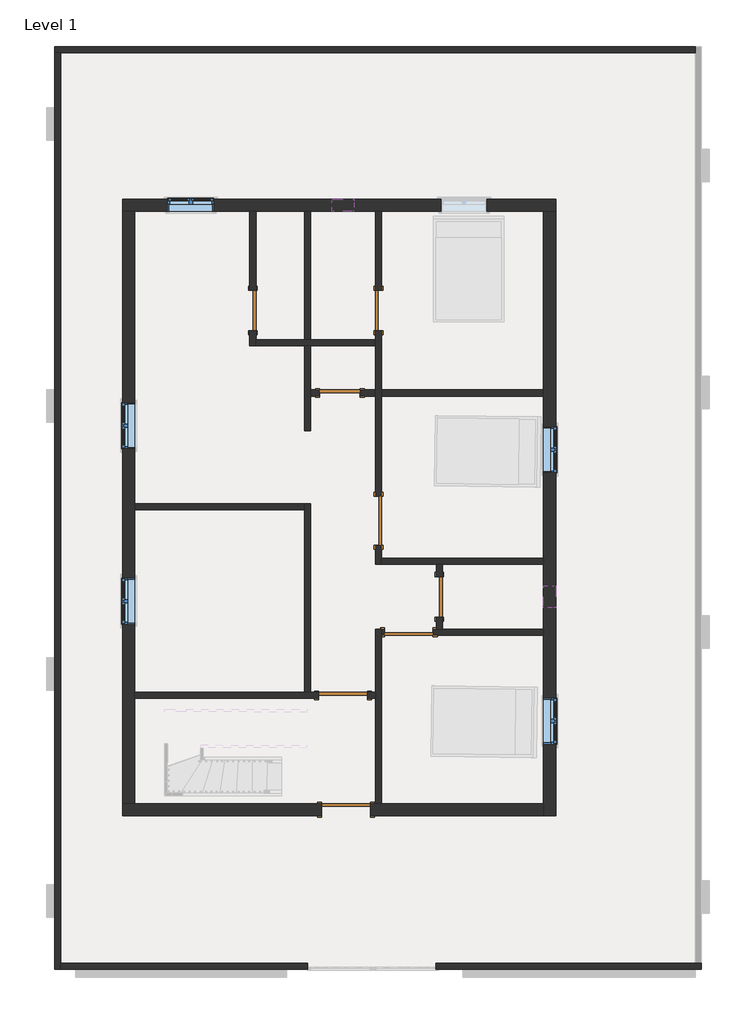
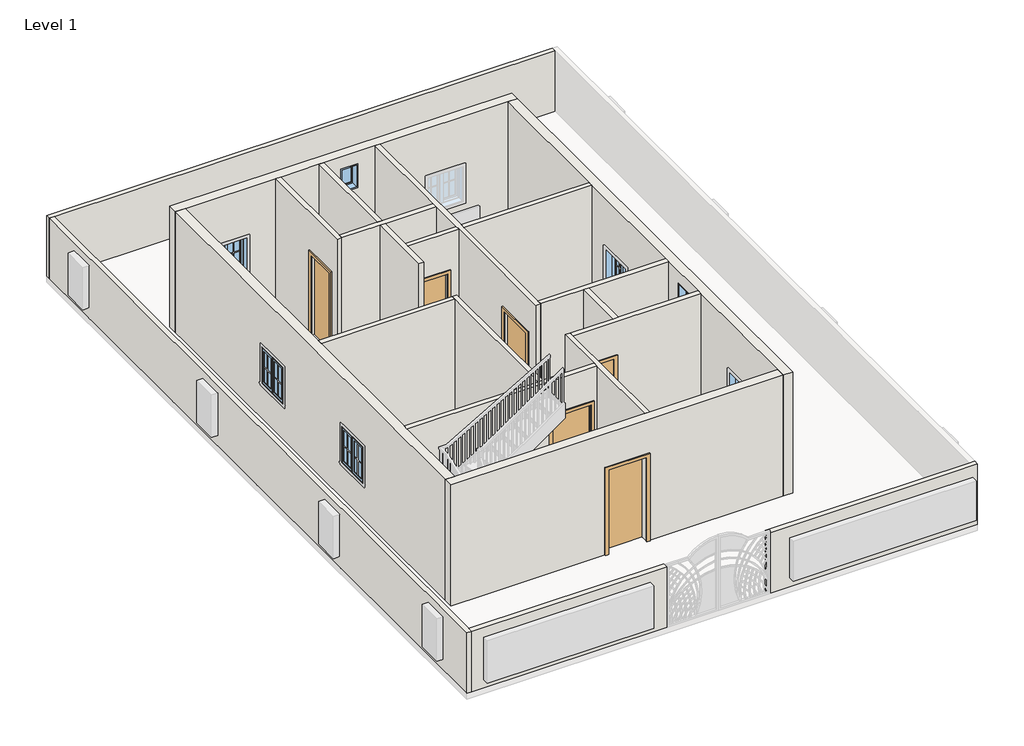
# One storey, part 1 of 3: 21 walls, 8 doors, 7 windows.
"""IFC4 building model written with IfcOpenShell, lengths in millimetres."""

from ifc_helpers import new_model, si_unit, frame, origin, origin_with_axes, place, context, project, spatial, polyline, outline, extrude, faceted_brep, transform, mapped, element, save
from components import door_d8f5dbb5, door_f2b275c1, door_e5f9f3c4, door_305aa2a5, door_0ca8825f, window_aa618e30, window_339605e1

model = new_model("IFC4")

# Units and contexts
model_context = context("Model", 3, world=origin())
ifc_project = project(units=[si_unit("LENGTHUNIT", "METRE", prefix="MILLI")], contexts=[model_context])

# Site, building, storey
site = spatial("IfcSite", under=ifc_project)
building = spatial("IfcBuilding", under=site)
storey = spatial("IfcBuildingStorey", under=building, Name="Level 1", Elevation=0.0)

# Doors
placement = place(None, origin())
door_shape = door_d8f5dbb5(model_context)
element("IfcDoor", 1, ObjectType="Single-Flush : 30\" x 80\"", at=placement, inside=storey, context=model_context, shape_type="MappedRepresentation", body=[
    mapped(door_shape, transform((-2883.8867314, 4242.0321212, 0.0), x_axis=(0.0, -1.0, 0.0), y_axis=(1.0, 0.0, 0.0), z_axis=(0.0, 0.0, 1.0))),
])
door_2_shape = door_f2b275c1(model_context)
element("IfcDoor", 2, ObjectType="Single-Flush : 30\" x 80\"", at=placement, inside=storey, context=model_context, shape_type="MappedRepresentation", body=[
    mapped(door_2_shape, transform((-521.6867314, 4242.0321212, 0.0), x_axis=(0.0, -1.0, 0.0), y_axis=(1.0, 0.0, 0.0), z_axis=(0.0, 0.0, 1.0))),
])
element("IfcDoor", 3, ObjectType="Single-Flush : 30\" x 80\"", at=placement, inside=storey, context=model_context, shape_type="MappedRepresentation", body=[
    mapped(door_2_shape, transform((-1245.5867314, 2692.6321212, 0.0), x_axis=(-1.0, 0.0, 0.0), y_axis=(0.0, -1.0, 0.0), z_axis=(0.0, 0.0, 1.0))),
])
element("IfcDoor", 4, ObjectType="Single-Flush : 30\" x 80\"", at=placement, inside=storey, context=model_context, shape_type="MappedRepresentation", body=[
    mapped(door_2_shape, transform((621.3132686, -1136.4178788, 0.0), x_axis=(0.0, 1.0, 0.0), y_axis=(-1.0, 0.0, 0.0), z_axis=(0.0, 0.0, 1.0))),
])
door_3_shape = door_e5f9f3c4(model_context)
element("IfcDoor", 5, ObjectType="Single-Flush : 36\" x 84\"", at=placement, inside=storey, context=model_context, shape_type="MappedRepresentation", body=[
    mapped(door_3_shape, transform((-521.6867314, 292.3321212, 0.0), x_axis=(0.0, -1.0, 0.0), y_axis=(1.0, 0.0, 0.0), z_axis=(0.0, 0.0, 1.0))),
])
element("IfcDoor", 6, ObjectType="Single-Flush : 36\" x 84\"", at=placement, inside=storey, context=model_context, shape_type="MappedRepresentation", body=[
    mapped(door_3_shape, transform((-1188.4367314, -2989.1542682, 0.0), x_axis=(1.0, 0.0, 0.0), y_axis=(0.0, 1.0, 0.0), z_axis=(0.0, 0.0, 1.0))),
])
door_4_shape = door_305aa2a5(model_context)
element("IfcDoor", 7, ObjectType="Single-Flush : 36\" x 84\"", at=placement, inside=storey, context=model_context, shape_type="MappedRepresentation", body=[
    mapped(door_4_shape, transform((49.8132686, -1803.1678788, 0.0), x_axis=(1.0, 0.0, 0.0), y_axis=(0.0, 1.0, 0.0), z_axis=(0.0, 0.0, 1.0))),
])
door_5_shape = door_0ca8825f(model_context)
element("IfcDoor", 8, ObjectType="Single-Flush : 36\" x 84\"", at=placement, inside=storey, context=model_context, shape_type="MappedRepresentation", body=[
    mapped(door_5_shape, transform((-1131.2867314, -5136.9178788, 0.0), x_axis=(1.0, 0.0, 0.0), y_axis=(0.0, 1.0, 0.0), z_axis=(0.0, 0.0, 1.0))),
])

# Walls
element("IfcWall", 9, ObjectType="wall4.5\"", at=placement, inside=storey, context=model_context, shape_type="Brep", body=[
    faceted_brep([(-2941.0367314, 3861.0321212, 2032.0), (-2941.0367314, 3861.0321212, 0.0), (-2941.0367314, 3575.2821212, 0.0), (-2941.0367314, 3575.2821212, 3048.0), (-2941.0367314, 6102.5821212, 3048.0), (-2941.0367314, 6102.5821212, 0.0), (-2941.0367314, 4623.0321212, 0.0), (-2941.0367314, 4623.0321212, 2032.0), (-2826.7367314, 3575.2821212, 0.0), (-2826.7367314, 3689.5821212, 0.0), (-2826.7367314, 3861.0321212, 0.0), (-2826.7367314, 3861.0321212, 2032.0), (-2826.7367314, 4623.0321212, 2032.0), (-2826.7367314, 4623.0321212, 0.0), (-2826.7367314, 6102.5821212, 0.0), (-2826.7367314, 6102.5821212, 3048.0), (-2826.7367314, 3689.5821212, 3048.0), (-2826.7367314, 3575.2821212, 3048.0)], [[[0, 1, 2, 3, 4, 5, 6, 7]], [[8, 9, 10, 11, 12, 13, 14, 15, 16, 17]], [[6, 5, 14, 13]], [[2, 1, 10, 9, 8]], [[4, 3, 17, 16, 15]], [[5, 4, 15, 14]], [[3, 2, 8, 17]], [[11, 10, 1, 0]], [[12, 11, 0, 7]], [[13, 12, 7, 6]]]),
])
element("IfcWall", 10, ObjectType="wall4.5\"", at=placement, inside=storey, context=model_context, shape_type="Brep", body=[
    faceted_brep([(-2826.7367314, 3575.2821212, 0.0), (-1912.3367314, 3575.2821212, 0.0), (-1798.0367314, 3575.2821212, 0.0), (-578.8367314, 3575.2821212, 0.0), (-578.8367314, 3575.2821212, 3048.0), (-1798.0367314, 3575.2821212, 3048.0), (-1912.3367314, 3575.2821212, 3048.0), (-2826.7367314, 3575.2821212, 3048.0), (-2826.7367314, 3689.5821212, 0.0), (-2826.7367314, 3689.5821212, 3048.0), (-1912.3367314, 3689.5821212, 3048.0), (-1798.0367314, 3689.5821212, 3048.0), (-578.8367314, 3689.5821212, 3048.0), (-578.8367314, 3689.5821212, 0.0), (-1798.0367314, 3689.5821212, 0.0), (-1912.3367314, 3689.5821212, 0.0)], [[[0, 1, 2, 3, 4, 5, 6, 7]], [[8, 9, 10, 11, 12, 13, 14, 15]], [[3, 2, 1, 0, 8, 15, 14, 13]], [[7, 6, 5, 4, 12, 11, 10, 9]], [[0, 7, 9, 8]], [[4, 3, 13, 12]]]),
])
element("IfcWall", 11, ObjectType="wall4.5\"", at=placement, inside=storey, context=model_context, shape_type="SweptSolid", body=[
    extrude(outline(polyline([(-1912.3367314, 3689.5821212), (-1912.3367314, 6102.5821212), (-1798.0367314, 6102.5821212), (-1798.0367314, 3689.5821212), (-1912.3367314, 3689.5821212)])), origin_with_axes(), (0.0, 0.0, 1.0), 3048.0),
])
element("IfcWall", 12, ObjectType="wall4.5\"", at=placement, inside=storey, context=model_context, shape_type="Brep", body=[
    faceted_brep([(-578.8367314, -164.8678788, 2133.6), (-578.8367314, -164.8678788, 0.0), (-578.8367314, -526.8178788, 0.0), (-578.8367314, -526.8178788, 3048.0), (-578.8367314, 2635.4821212, 3048.0), (-578.8367314, 2749.7821212, 3048.0), (-578.8367314, 3575.2821212, 3048.0), (-578.8367314, 3689.5821212, 3048.0), (-578.8367314, 6102.5821212, 3048.0), (-578.8367314, 6102.5821212, 0.0), (-578.8367314, 4623.0321212, 0.0), (-578.8367314, 4623.0321212, 2032.0), (-578.8367314, 3861.0321212, 2032.0), (-578.8367314, 3861.0321212, 0.0), (-578.8367314, 3689.5821212, 0.0), (-578.8367314, 3575.2821212, 0.0), (-578.8367314, 2749.7821212, 0.0), (-578.8367314, 2635.4821212, 0.0), (-578.8367314, 749.5321212, 0.0), (-578.8367314, 749.5321212, 2133.6), (-464.5367314, -526.8178788, 0.0), (-464.5367314, -412.5178788, 0.0), (-464.5367314, -164.8678788, 0.0), (-464.5367314, -164.8678788, 2133.6), (-464.5367314, 749.5321212, 2133.6), (-464.5367314, 749.5321212, 0.0), (-464.5367314, 2635.4821212, 0.0), (-464.5367314, 2749.7821212, 0.0), (-464.5367314, 3861.0321212, 0.0), (-464.5367314, 3861.0321212, 2032.0), (-464.5367314, 4623.0321212, 2032.0), (-464.5367314, 4623.0321212, 0.0), (-464.5367314, 6102.5821212, 0.0), (-464.5367314, 6102.5821212, 3048.0), (-464.5367314, 2749.7821212, 3048.0), (-464.5367314, 2635.4821212, 3048.0), (-464.5367314, -412.5178788, 3048.0), (-464.5367314, -526.8178788, 3048.0)], [[[0, 1, 2, 3, 4, 5, 6, 7, 8, 9, 10, 11, 12, 13, 14, 15, 16, 17, 18, 19]], [[20, 21, 22, 23, 24, 25, 26, 27, 28, 29, 30, 31, 32, 33, 34, 35, 36, 37]], [[10, 9, 32, 31]], [[2, 1, 22, 21, 20]], [[18, 17, 16, 15, 14, 13, 28, 27, 26, 25]], [[8, 7, 6, 5, 4, 3, 37, 36, 35, 34, 33]], [[9, 8, 33, 32]], [[3, 2, 20, 37]], [[29, 28, 13, 12]], [[30, 29, 12, 11]], [[31, 30, 11, 10]], [[23, 22, 1, 0]], [[24, 23, 0, 19]], [[25, 24, 19, 18]]]),
])
element("IfcWall", 13, ObjectType="wall4.5\"", at=placement, inside=storey, context=model_context, shape_type="Brep", body=[
    faceted_brep([(-464.5367314, -526.8178788, 0.0), (564.1632686, -526.8178788, 0.0), (678.4632686, -526.8178788, 0.0), (2583.4632686, -526.8178788, 0.0), (2583.4632686, -526.8178788, 3048.0), (678.4632686, -526.8178788, 3048.0), (564.1632686, -526.8178788, 3048.0), (-464.5367314, -526.8178788, 3048.0), (-464.5367314, -412.5178788, 0.0), (-464.5367314, -412.5178788, 3048.0), (2583.4632686, -412.5178788, 3048.0), (2583.4632686, -412.5178788, 0.0)], [[[0, 1, 2, 3, 4, 5, 6, 7]], [[8, 9, 10, 11]], [[3, 2, 1, 0, 8, 11]], [[7, 6, 5, 4, 10, 9]], [[0, 7, 9, 8]], [[4, 3, 11, 10]]]),
])
element("IfcWall", 14, ObjectType="wall4.5\"", at=placement, inside=storey, context=model_context, shape_type="SweptSolid", body=[
    extrude(outline(polyline([(2583.4632686, 2749.7821212), (2583.4632686, 2635.4821212), (-464.5367314, 2635.4821212), (-464.5367314, 2749.7821212), (2583.4632686, 2749.7821212)])), origin_with_axes(), (0.0, 0.0, 1.0), 3048.0),
    extrude(outline(polyline([(3048.0, -1798.0367314), (0.0, -1798.0367314), (0.0, -1626.5867314), (2032.0, -1626.5867314), (2032.0, -864.5867314), (0.0, -864.5867314), (0.0, -578.8367314), (3048.0, -578.8367314), (3048.0, -1798.0367314)])), frame((0.0, 2635.4821212, 0.0), z_axis=(0.0, 1.0, 0.0), x_axis=(0.0, 0.0, 1.0)), (0.0, 0.0, 1.0), 114.3),
])
element("IfcWall", 15, ObjectType="wall4.5\"", at=placement, inside=storey, context=model_context, shape_type="Brep", body=[
    faceted_brep([(-1912.3367314, 3575.2821212, 0.0), (-1912.3367314, 1982.8957318, 0.0), (-1912.3367314, 1982.8957318, 3048.0), (-1912.3367314, 3575.2821212, 3048.0), (-1798.0367314, 3575.2821212, 0.0), (-1798.0367314, 3575.2821212, 3048.0), (-1798.0367314, 2749.7821212, 3048.0), (-1798.0367314, 2635.4821212, 3048.0), (-1798.0367314, 1982.8957318, 3048.0), (-1798.0367314, 1982.8957318, 0.0), (-1798.0367314, 2635.4821212, 0.0), (-1798.0367314, 2749.7821212, 0.0)], [[[0, 1, 2, 3]], [[4, 5, 6, 7, 8, 9, 10, 11]], [[1, 0, 4, 11, 10, 9]], [[2, 1, 9, 8]], [[3, 2, 8, 7, 6, 5]], [[0, 3, 5, 4]]]),
])
element("IfcWall", 16, ObjectType="wall4.5\"", at=placement, inside=storey, context=model_context, shape_type="Brep", body=[
    faceted_brep([(-1912.3367314, 611.2957318, 0.0), (-1912.3367314, 496.9957318, 0.0), (-1912.3367314, -2932.0042682, 0.0), (-1912.3367314, -2932.0042682, 3048.0), (-1912.3367314, 496.9957318, 3048.0), (-1912.3367314, 611.2957318, 3048.0), (-1798.0367314, 611.2957318, 0.0), (-1798.0367314, 611.2957318, 3048.0), (-1798.0367314, -2932.0042682, 3048.0), (-1798.0367314, -2932.0042682, 0.0)], [[[0, 1, 2, 3, 4, 5]], [[6, 7, 8, 9]], [[2, 1, 0, 6, 9]], [[5, 4, 3, 8, 7]], [[3, 2, 9, 8]], [[0, 5, 7, 6]]]),
])
element("IfcWall", 17, ObjectType="wall4.5\"", at=placement, inside=storey, context=model_context, shape_type="Brep", body=[
    faceted_brep([(-731.2367314, -3046.3042682, 2133.6), (-731.2367314, -3046.3042682, 0.0), (-578.8367314, -3046.3042682, 0.0), (-578.8367314, -3046.3042682, 3048.0), (-5100.0367314, -3046.3042682, 3048.0), (-5100.0367314, -3046.3042682, 0.0), (-1645.6367314, -3046.3042682, 0.0), (-1645.6367314, -3046.3042682, 2133.6), (-578.8367314, -2932.0042682, 0.0), (-731.2367314, -2932.0042682, 0.0), (-731.2367314, -2932.0042682, 2133.6), (-1645.6367314, -2932.0042682, 2133.6), (-1645.6367314, -2932.0042682, 0.0), (-1798.0367314, -2932.0042682, 0.0), (-1912.3367314, -2932.0042682, 0.0), (-5100.0367314, -2932.0042682, 0.0), (-5100.0367314, -2932.0042682, 3048.0), (-1912.3367314, -2932.0042682, 3048.0), (-1798.0367314, -2932.0042682, 3048.0), (-578.8367314, -2932.0042682, 3048.0)], [[[0, 1, 2, 3, 4, 5, 6, 7]], [[8, 9, 10, 11, 12, 13, 14, 15, 16, 17, 18, 19]], [[6, 5, 15, 14, 13, 12]], [[2, 1, 9, 8]], [[4, 3, 19, 18, 17, 16]], [[5, 4, 16, 15]], [[3, 2, 8, 19]], [[10, 9, 1, 0]], [[11, 10, 0, 7]], [[12, 11, 7, 6]]]),
])
element("IfcWall", 18, ObjectType="wall4.5\"", at=placement, inside=storey, context=model_context, shape_type="Brep", body=[
    faceted_brep([(-464.5367314, -5022.6178788, 0.0), (-464.5367314, -1860.3178788, 0.0), (-464.5367314, -1746.0178788, 0.0), (-464.5367314, -1746.0178788, 3048.0), (-464.5367314, -1860.3178788, 3048.0), (-464.5367314, -5022.6178788, 3048.0), (-578.8367314, -5022.6178788, 0.0), (-578.8367314, -5022.6178788, 3048.0), (-578.8367314, -3046.3042682, 3048.0), (-578.8367314, -2932.0042682, 3048.0), (-578.8367314, -1746.0178788, 3048.0), (-578.8367314, -1746.0178788, 0.0), (-578.8367314, -2932.0042682, 0.0), (-578.8367314, -3046.3042682, 0.0)], [[[0, 1, 2, 3, 4, 5]], [[6, 7, 8, 9, 10, 11, 12, 13]], [[2, 1, 0, 6, 13, 12, 11]], [[5, 4, 3, 10, 9, 8, 7]], [[0, 5, 7, 6]], [[3, 2, 11, 10]]]),
])
element("IfcWall", 19, ObjectType="wall4.5\"", at=placement, inside=storey, context=model_context, shape_type="Brep", body=[
    faceted_brep([(507.0132686, -1860.3178788, 2133.6), (507.0132686, -1860.3178788, 0.0), (2583.4632686, -1860.3178788, 0.0), (2583.4632686, -1860.3178788, 3048.0), (-464.5367314, -1860.3178788, 3048.0), (-464.5367314, -1860.3178788, 0.0), (-407.3867314, -1860.3178788, 0.0), (-407.3867314, -1860.3178788, 2133.6), (2583.4632686, -1746.0178788, 0.0), (678.4632686, -1746.0178788, 0.0), (564.1632686, -1746.0178788, 0.0), (507.0132686, -1746.0178788, 0.0), (507.0132686, -1746.0178788, 2133.6), (-407.3867314, -1746.0178788, 2133.6), (-407.3867314, -1746.0178788, 0.0), (-464.5367314, -1746.0178788, 0.0), (-464.5367314, -1746.0178788, 3048.0), (564.1632686, -1746.0178788, 3048.0), (678.4632686, -1746.0178788, 3048.0), (2583.4632686, -1746.0178788, 3048.0)], [[[0, 1, 2, 3, 4, 5, 6, 7]], [[8, 9, 10, 11, 12, 13, 14, 15, 16, 17, 18, 19]], [[6, 5, 15, 14]], [[2, 1, 11, 10, 9, 8]], [[4, 3, 19, 18, 17, 16]], [[5, 4, 16, 15]], [[3, 2, 8, 19]], [[12, 11, 1, 0]], [[13, 12, 0, 7]], [[14, 13, 7, 6]]]),
])
element("IfcWall", 20, ObjectType="wall4.5\"", at=placement, inside=storey, context=model_context, shape_type="SweptSolid", body=[
    extrude(outline(polyline([(-526.8178788, 0.0), (-755.4178788, 0.0), (-755.4178788, 2032.0), (-1517.4178788, 2032.0), (-1517.4178788, 0.0), (-1746.0178788, 0.0), (-1746.0178788, 3048.0), (-526.8178788, 3048.0), (-526.8178788, 0.0)])), frame((564.1632686, 0.0, 0.0), z_axis=(1.0, 0.0, 0.0), x_axis=(0.0, 1.0, 0.0)), (0.0, 0.0, 1.0), 114.3),
])
element("IfcWall", 21, ObjectType="wall4.5\"", at=placement, inside=storey, context=model_context, shape_type="SweptSolid", body=[
    extrude(outline(polyline([(-5100.0367314, 611.2957318), (-1912.3367314, 611.2957318), (-1912.3367314, 496.9957318), (-5100.0367314, 496.9957318), (-5100.0367314, 611.2957318)])), origin_with_axes(), (0.0, 0.0, 1.0), 3048.0),
])
element("IfcWall", 22, ObjectType="wall4.5\"", at=placement, inside=storey, context=model_context, shape_type="Brep", body=[
    faceted_brep([(-6609.1977342, 9086.2938411, 0.0), (-6494.8977342, 9086.2938411, 0.0), (5430.4022658, 9086.2938411, 0.0), (5430.4022658, 9086.2938411, 1524.0), (-6494.8977342, 9086.2938411, 1524.0), (-6609.1977342, 9086.2938411, 1524.0), (-6609.1977342, 9200.5938411, 0.0), (-6609.1977342, 9200.5938411, 1524.0), (5430.4022658, 9200.5938411, 1524.0), (5430.4022658, 9200.5938411, 0.0)], [[[0, 1, 2, 3, 4, 5]], [[6, 7, 8, 9]], [[2, 1, 0, 6, 9]], [[5, 4, 3, 8, 7]], [[0, 5, 7, 6]], [[3, 2, 9, 8]]]),
])
element("IfcWall", 23, ObjectType="wall4.5\"", at=placement, inside=storey, context=model_context, shape_type="Brep", body=[
    faceted_brep([(-6494.8977342, -8134.9061589, 0.0), (-6494.8977342, -8020.6061589, 0.0), (-6494.8977342, 9086.2938411, 0.0), (-6494.8977342, 9086.2938411, 1524.0), (-6494.8977342, -8020.6061589, 1524.0), (-6494.8977342, -8134.9061589, 1524.0), (-6609.1977342, -8134.9061589, 0.0), (-6609.1977342, -8134.9061589, 1524.0), (-6609.1977342, 9086.2938411, 1524.0), (-6609.1977342, 9086.2938411, 0.0)], [[[0, 1, 2, 3, 4, 5]], [[6, 7, 8, 9]], [[2, 1, 0, 6, 9]], [[5, 4, 3, 8, 7]], [[0, 5, 7, 6]], [[3, 2, 9, 8]]]),
])
element("IfcWall", 24, ObjectType="wall4.5\"", at=placement, inside=storey, context=model_context, shape_type="Brep", body=[
    faceted_brep([(5544.7022658, -8020.6061589, 0.0), (5430.4022658, -8020.6061589, 0.0), (559.9522658, -8020.6061589, 0.0), (559.9522658, -8020.6061589, 1524.0), (5430.4022658, -8020.6061589, 1524.0), (5544.7022658, -8020.6061589, 1524.0), (5544.7022658, -8134.9061589, 0.0), (5544.7022658, -8134.9061589, 1524.0), (559.9522658, -8134.9061589, 1524.0), (559.9522658, -8134.9061589, 0.0)], [[[0, 1, 2, 3, 4, 5]], [[6, 7, 8, 9]], [[2, 1, 0, 6, 9]], [[3, 2, 9, 8]], [[5, 4, 3, 8, 7]], [[0, 5, 7, 6]]]),
])
element("IfcWall", 25, ObjectType="wall4.5\"", at=placement, inside=storey, context=model_context, shape_type="SweptSolid", body=[
    extrude(outline(polyline([(-6494.8977342, -8020.6061589), (-1853.0477342, -8020.6061589), (-1853.0477342, -8134.9061589), (-6494.8977342, -8134.9061589), (-6494.8977342, -8020.6061589)])), origin_with_axes(), (0.0, 0.0, 1.0), 1524.0),
])
element("IfcWall", 26, ObjectType="wall9\"", at=placement, inside=storey, context=model_context, shape_type="Brep", body=[
    faceted_brep([(-5328.6367314, 6102.5821212, 0.0), (-5100.0367314, 6102.5821212, 0.0), (-2941.0367314, 6102.5821212, 0.0), (-2826.7367314, 6102.5821212, 0.0), (-1912.3367314, 6102.5821212, 0.0), (-1798.0367314, 6102.5821212, 0.0), (-578.8367314, 6102.5821212, 0.0), (-464.5367314, 6102.5821212, 0.0), (2583.4632686, 6102.5821212, 0.0), (2812.0632686, 6102.5821212, 0.0), (2812.0632686, 6102.5821212, 3048.0), (2583.4632686, 6102.5821212, 3048.0), (-464.5367314, 6102.5821212, 3048.0), (-578.8367314, 6102.5821212, 3048.0), (-1798.0367314, 6102.5821212, 3048.0), (-1912.3367314, 6102.5821212, 3048.0), (-2826.7367314, 6102.5821212, 3048.0), (-2941.0367314, 6102.5821212, 3048.0), (-5100.0367314, 6102.5821212, 3048.0), (-5328.6367314, 6102.5821212, 3048.0), (-985.2367314, 6102.5821212, 2743.2), (-985.2367314, 6102.5821212, 2133.6), (-1391.6367314, 6102.5821212, 2133.6), (-1391.6367314, 6102.5821212, 2743.2), (1519.8382686, 6102.5821212, 1828.8), (1519.8382686, 6102.5821212, 914.4), (656.2382686, 6102.5821212, 914.4), (656.2382686, 6102.5821212, 1828.8), (-3617.3117314, 6102.5821212, 1828.8), (-3617.3117314, 6102.5821212, 914.4), (-4480.9117314, 6102.5821212, 914.4), (-4480.9117314, 6102.5821212, 1828.8), (-5328.6367314, 6331.1821212, 0.0), (-5328.6367314, 6331.1821212, 3048.0), (2812.0632686, 6331.1821212, 3048.0), (2812.0632686, 6331.1821212, 0.0), (-985.2367314, 6331.1821212, 2743.2), (-1391.6367314, 6331.1821212, 2743.2), (-1391.6367314, 6331.1821212, 2133.6), (-985.2367314, 6331.1821212, 2133.6), (1519.8382686, 6331.1821212, 1828.8), (656.2382686, 6331.1821212, 1828.8), (656.2382686, 6331.1821212, 914.4), (1519.8382686, 6331.1821212, 914.4), (-3617.3117314, 6331.1821212, 1828.8), (-4480.9117314, 6331.1821212, 1828.8), (-4480.9117314, 6331.1821212, 914.4), (-3617.3117314, 6331.1821212, 914.4)], [[[0, 1, 2, 3, 4, 5, 6, 7, 8, 9, 10, 11, 12, 13, 14, 15, 16, 17, 18, 19], [20, 21, 22, 23], [24, 25, 26, 27], [28, 29, 30, 31]], [[32, 33, 34, 35], [36, 37, 38, 39], [40, 41, 42, 43], [44, 45, 46, 47]], [[9, 8, 7, 6, 5, 4, 3, 2, 1, 0, 32, 35]], [[19, 18, 17, 16, 15, 14, 13, 12, 11, 10, 34, 33]], [[10, 9, 35, 34]], [[0, 19, 33, 32]], [[21, 20, 36, 39]], [[22, 21, 39, 38]], [[23, 22, 38, 37]], [[20, 23, 37, 36]], [[25, 24, 40, 43]], [[26, 25, 43, 42]], [[27, 26, 42, 41]], [[24, 27, 41, 40]], [[29, 28, 44, 47]], [[30, 29, 47, 46]], [[31, 30, 46, 45]], [[28, 31, 45, 44]]]),
])
element("IfcWall", 27, ObjectType="wall9\"", at=placement, inside=storey, context=model_context, shape_type="Brep", body=[
    faceted_brep([(2583.4632686, 6102.5821212, 0.0), (2583.4632686, 2749.7821212, 0.0), (2583.4632686, 2635.4821212, 0.0), (2583.4632686, -412.5178788, 0.0), (2583.4632686, -526.8178788, 0.0), (2583.4632686, -1746.0178788, 0.0), (2583.4632686, -1860.3178788, 0.0), (2583.4632686, -5022.6178788, 0.0), (2583.4632686, -5251.2178788, 0.0), (2583.4632686, -5251.2178788, 3048.0), (2583.4632686, -5022.6178788, 3048.0), (2583.4632686, -1860.3178788, 3048.0), (2583.4632686, -1746.0178788, 3048.0), (2583.4632686, -526.8178788, 3048.0), (2583.4632686, -412.5178788, 3048.0), (2583.4632686, 2635.4821212, 3048.0), (2583.4632686, 2749.7821212, 3048.0), (2583.4632686, 6102.5821212, 3048.0), (2583.4632686, -1339.6178788, 2743.2), (2583.4632686, -1339.6178788, 2133.6), (2583.4632686, -933.2178788, 2133.6), (2583.4632686, -933.2178788, 2743.2), (2583.4632686, 1194.0321212, 1828.8), (2583.4632686, 1194.0321212, 914.4), (2583.4632686, 2057.6321212, 914.4), (2583.4632686, 2057.6321212, 1828.8), (2583.4632686, -3901.8428788, 1828.8), (2583.4632686, -3901.8428788, 914.4), (2583.4632686, -3038.2428788, 914.4), (2583.4632686, -3038.2428788, 1828.8), (2812.0632686, 6102.5821212, 0.0), (2812.0632686, 6102.5821212, 3048.0), (2812.0632686, -5251.2178788, 3048.0), (2812.0632686, -5251.2178788, 0.0), (2812.0632686, -1339.6178788, 2743.2), (2812.0632686, -933.2178788, 2743.2), (2812.0632686, -933.2178788, 2133.6), (2812.0632686, -1339.6178788, 2133.6), (2812.0632686, 1194.0321212, 1828.8), (2812.0632686, 2057.6321212, 1828.8), (2812.0632686, 2057.6321212, 914.4), (2812.0632686, 1194.0321212, 914.4), (2812.0632686, -3901.8428788, 1828.8), (2812.0632686, -3038.2428788, 1828.8), (2812.0632686, -3038.2428788, 914.4), (2812.0632686, -3901.8428788, 914.4)], [[[0, 1, 2, 3, 4, 5, 6, 7, 8, 9, 10, 11, 12, 13, 14, 15, 16, 17], [18, 19, 20, 21], [22, 23, 24, 25], [26, 27, 28, 29]], [[30, 31, 32, 33], [34, 35, 36, 37], [38, 39, 40, 41], [42, 43, 44, 45]], [[8, 7, 6, 5, 4, 3, 2, 1, 0, 30, 33]], [[17, 16, 15, 14, 13, 12, 11, 10, 9, 32, 31]], [[0, 17, 31, 30]], [[9, 8, 33, 32]], [[19, 18, 34, 37]], [[20, 19, 37, 36]], [[21, 20, 36, 35]], [[18, 21, 35, 34]], [[23, 22, 38, 41]], [[24, 23, 41, 40]], [[25, 24, 40, 39]], [[22, 25, 39, 38]], [[27, 26, 42, 45]], [[28, 27, 45, 44]], [[29, 28, 44, 43]], [[26, 29, 43, 42]]]),
])
element("IfcWall", 28, ObjectType="wall9\"", at=placement, inside=storey, context=model_context, shape_type="Brep", body=[
    faceted_brep([(2583.4632686, -5022.6178788, 0.0), (-464.5367314, -5022.6178788, 0.0), (-578.8367314, -5022.6178788, 0.0), (-674.0867314, -5022.6178788, 0.0), (-674.0867314, -5022.6178788, 2133.6), (-1588.4867314, -5022.6178788, 2133.6), (-1588.4867314, -5022.6178788, 0.0), (-5100.0367314, -5022.6178788, 0.0), (-5328.6367314, -5022.6178788, 0.0), (-5328.6367314, -5022.6178788, 3048.0), (-5100.0367314, -5022.6178788, 3048.0), (-578.8367314, -5022.6178788, 3048.0), (-464.5367314, -5022.6178788, 3048.0), (2583.4632686, -5022.6178788, 3048.0), (-674.0867314, -5251.2178788, 2133.6), (-674.0867314, -5251.2178788, 0.0), (2583.4632686, -5251.2178788, 0.0), (2583.4632686, -5251.2178788, 3048.0), (-5328.6367314, -5251.2178788, 3048.0), (-5328.6367314, -5251.2178788, 0.0), (-1588.4867314, -5251.2178788, 0.0), (-1588.4867314, -5251.2178788, 2133.6)], [[[0, 1, 2, 3, 4, 5, 6, 7, 8, 9, 10, 11, 12, 13]], [[14, 15, 16, 17, 18, 19, 20, 21]], [[20, 19, 8, 7, 6]], [[16, 15, 3, 2, 1, 0]], [[13, 12, 11, 10, 9, 18, 17]], [[0, 13, 17, 16]], [[9, 8, 19, 18]], [[4, 3, 15, 14]], [[5, 4, 14, 21]], [[6, 5, 21, 20]]]),
])
element("IfcWall", 29, ObjectType="wall9\"", at=placement, inside=storey, context=model_context, shape_type="Brep", body=[
    faceted_brep([(-5328.6367314, 6102.5821212, 0.0), (-5328.6367314, -5022.6178788, 0.0), (-5328.6367314, -5022.6178788, 3048.0), (-5328.6367314, 6102.5821212, 3048.0), (-5328.6367314, 2509.9457318, 1828.8), (-5328.6367314, 1646.3457318, 1828.8), (-5328.6367314, 1646.3457318, 914.4), (-5328.6367314, 2509.9457318, 914.4), (-5328.6367314, -785.7042682, 1828.8), (-5328.6367314, -1649.3042682, 1828.8), (-5328.6367314, -1649.3042682, 914.4), (-5328.6367314, -785.7042682, 914.4), (-5100.0367314, 6102.5821212, 0.0), (-5100.0367314, 6102.5821212, 3048.0), (-5100.0367314, 611.2957318, 3048.0), (-5100.0367314, 496.9957318, 3048.0), (-5100.0367314, -2932.0042682, 3048.0), (-5100.0367314, -3046.3042682, 3048.0), (-5100.0367314, -5022.6178788, 3048.0), (-5100.0367314, -5022.6178788, 0.0), (-5100.0367314, -3046.3042682, 0.0), (-5100.0367314, -2932.0042682, 0.0), (-5100.0367314, 496.9957318, 0.0), (-5100.0367314, 611.2957318, 0.0), (-5100.0367314, 2509.9457318, 1828.8), (-5100.0367314, 2509.9457318, 914.4), (-5100.0367314, 1646.3457318, 914.4), (-5100.0367314, 1646.3457318, 1828.8), (-5100.0367314, -785.7042682, 1828.8), (-5100.0367314, -785.7042682, 914.4), (-5100.0367314, -1649.3042682, 914.4), (-5100.0367314, -1649.3042682, 1828.8)], [[[0, 1, 2, 3], [4, 5, 6, 7], [8, 9, 10, 11]], [[12, 13, 14, 15, 16, 17, 18, 19, 20, 21, 22, 23], [24, 25, 26, 27], [28, 29, 30, 31]], [[1, 0, 12, 23, 22, 21, 20, 19]], [[3, 2, 18, 17, 16, 15, 14, 13]], [[0, 3, 13, 12]], [[2, 1, 19, 18]], [[25, 24, 4, 7]], [[26, 25, 7, 6]], [[27, 26, 6, 5]], [[24, 27, 5, 4]], [[29, 28, 8, 11]], [[30, 29, 11, 10]], [[31, 30, 10, 9]], [[28, 31, 9, 8]]]),
])

# Windows
window_shape = window_aa618e30(model_context)
element("IfcWindow", 30, ObjectType="Fixed : 16\" x 24\"", at=placement, inside=storey, context=model_context, shape_type="MappedRepresentation", body=[
    mapped(window_shape, transform((-1150.3367314, 6216.8821212, 1219.2), x_axis=(1.0, 0.0, 0.0), y_axis=(0.0, 1.0, 0.0), z_axis=(0.0, 0.0, 1.0))),
])
element("IfcWindow", 31, ObjectType="Fixed : 16\" x 24\"", at=placement, inside=storey, context=model_context, shape_type="MappedRepresentation", body=[
    mapped(window_shape, transform((2697.7632686, -1174.5178788, 1219.2), x_axis=(0.0, -1.0, 0.0), y_axis=(1.0, 0.0, 0.0), z_axis=(0.0, 0.0, 1.0))),
])
window_2_shape = window_339605e1(model_context)
element("IfcWindow", 32, ObjectType="Window-Casement-Double : 34\" x 36\"", at=placement, inside=storey, context=model_context, shape_type="MappedRepresentation", body=[
    mapped(window_2_shape, transform((2697.7632686, 1625.8321212, 0.0), x_axis=(0.0, -1.0, 0.0), y_axis=(1.0, 0.0, 0.0), z_axis=(0.0, 0.0, 1.0))),
])
element("IfcWindow", 33, ObjectType="Window-Casement-Double : 34\" x 36\"", at=placement, inside=storey, context=model_context, shape_type="MappedRepresentation", body=[
    mapped(window_2_shape, transform((2697.7632686, -3470.0428788, 0.0), x_axis=(0.0, -1.0, 0.0), y_axis=(1.0, 0.0, 0.0), z_axis=(0.0, 0.0, 1.0))),
])
element("IfcWindow", 34, ObjectType="Window-Casement-Double : 34\" x 36\"", at=placement, inside=storey, context=model_context, shape_type="MappedRepresentation", body=[
    mapped(window_2_shape, transform((-4049.1117314, 6216.8821212, 0.0), x_axis=(1.0, 0.0, 0.0), y_axis=(0.0, 1.0, 0.0), z_axis=(0.0, 0.0, 1.0))),
])
element("IfcWindow", 35, ObjectType="Window-Casement-Double : 34\" x 36\"", at=placement, inside=storey, context=model_context, shape_type="MappedRepresentation", body=[
    mapped(window_2_shape, transform((-5214.3367314, 2078.1457318, 0.0), x_axis=(0.0, 1.0, 0.0), y_axis=(-1.0, 0.0, 0.0), z_axis=(0.0, 0.0, 1.0))),
])
element("IfcWindow", 36, ObjectType="Window-Casement-Double : 34\" x 36\"", at=placement, inside=storey, context=model_context, shape_type="MappedRepresentation", body=[
    mapped(window_2_shape, transform((-5214.3367314, -1217.5042682, 0.0), x_axis=(0.0, 1.0, 0.0), y_axis=(-1.0, 0.0, 0.0), z_axis=(0.0, 0.0, 1.0))),
])

save(model, "model.ifc")

# Revit data of these elements
# Type "Single-Flush : 30\" x 80\""
#   Type Mark = "5"
#   Construction Type Id = "MDOOR"
#   Assembly Code = "C1020"
#   Analytic Construction = "Metal"
#   Thickness = 0' - 2"
#   Heat Transfer Coefficient (U) = 0.651978 BTU/(h·ft²·°F)
#   Height = 6' - 8"
#   Trim Projection Ext = 0' - 1"
#   Trim Projection Int = 0' - 1"
#   Trim Width = 0' - 3"
#   Width = 2' - 6"
#   Define Thermal Properties by = 1
#   Define Thermal Properties by = 1
#   Door Material = Door - Panel
#   Frame Material = Door - Frame
#   Visual Light Transmittance = 0
#   Solar Heat Gain Coefficient = 0
#   Function = (empty or 0)
#   Wall Closure = (empty or 0)
# Type "Single-Flush : 36\" x 84\""
#   Type Mark = "1"
#   Construction Type Id = "MDOOR"
#   Assembly Code = "C1020"
#   Analytic Construction = "Metal"
#   Thickness = 0' - 2"
#   Heat Transfer Coefficient (U) = 0.651978 BTU/(h·ft²·°F)
#   Height = 7' - 0"
#   Trim Projection Ext = 0' - 1"
#   Trim Projection Int = 0' - 1"
#   Trim Width = 0' - 3"
#   Width = 3' - 0"
#   Define Thermal Properties by = 1
#   Define Thermal Properties by = 1
#   Door Material = Door - Panel
#   Frame Material = Door - Frame
#   Visual Light Transmittance = 0
#   Solar Heat Gain Coefficient = 0
#   Function = (empty or 0)
#   Wall Closure = (empty or 0)
# Type "wall4.5\""
#   Assembly Code = "B2010"
#   Layers, outside or top first: 0' - 4 1/2" no material (function 1)
# Type "wall9\""
#   Assembly Code = "B2010"
#   Layers, outside or top first: 0' - 9" no material (function 1)
# Type "Fixed : 16\" x 24\""
#   Type Mark = "4"
#   Construction Type Id = "GSP4R"
#   Assembly Code = "B2020100"
#   Analytic Construction = "1/8 in Pilkington single glazing"
#   Visual Light Transmittance = 0.9
#   Solar Heat Gain Coefficient = 0.78
#   Heat Transfer Coefficient (U) = 0.6496 BTU/(h·ft²·°F)
#   Height = 2' - 0"
#   Default Sill Height = 3' - 0"
#   Width = 1' - 4"
#   Window Inset = 0' - 0 3/4"
#   Define Thermal Properties by = 1
#   Define Thermal Properties by = 1
#   Glass Pane Material = Glass
#   Sash Material = Sash
#   Wall Closure = (empty or 0)
# Type "Window-Casement-Double : 34\" x 36\""
#   Type Mark = "14"
#   Fire Rating = "0.5h"
#   Assembly Code = "B2020100"
#   Analytic Construction = "Double glazing - domestic"
#   Frame Extension [instance default] = 0' - 0 1/4"
#   Window Inset [instance default] = 0' - 0"
#   Wall Thickness [instance default] = 0' - 6"
#   Interior Wall Closure [instance default] = 0' - 2 1/4"
#   Half Width = 1' - 5"
#   Visual Light Transmittance = 0.81
#   Thermal Resistance (R) = 1.8146 (h·ft²·°F)/BTU
#   Solar Heat Gain Coefficient = 0.76
#   Rough Width = 2' - 10 1/2"
#   Rough Height = 3' - 0 1/2"
#   Height = 3' - 0"
#   Heat Transfer Coefficient (U) = 0.5511 BTU/(h·ft²·°F)
#   Exterior Wall Closure [instance default] = 0' - 1 1/4"
#   Extension Jamb [instance default] = 0' - 2 1/4"
#   Default Sill Height = 3' - 0"
#   Width = 2' - 10"
#   Define Thermal Properties by = 0
#   Muntin Visibility = yes
#   Interior Trim Visibility [instance default] = yes
#   Exterior Trim Visibility [instance default] = yes
#   Extension Jamb Visibility [instance default] = yes
#   Interior Trim Material = Wood - Stained
#   Muntin Pattern = Muntin Pattern_2x2 : Muntin Pattern_2x2
#   Interior Trim = Trim-Window-Interior-Flat : Picture Frame
#   Interior Frame Material = Wood - Stained
#   Glass Panel Material = Glass
#   Exterior Trim Material = Clad - White
#   Exterior Trim = Trim-Window-Exterior-Flat : with Sill
#   Exterior Frame Material = Clad - White
#   Wall Closure = (empty or 0)
# Elements 1, 2, 3, 4 (IfcDoor, "Single-Flush : 30\" x 80\"")
#   Phase Created = New Construction
#   Materials on its faces: "Door - Frame", "Door - Panel"
# Elements 5, 6, 7, 8 (IfcDoor, "Single-Flush : 36\" x 84\"")
#   Phase Created = New Construction
#   Materials on its faces: "Door - Frame", "Door - Panel"
# Elements 9, 10, 11, 12, 13, 14, 15, 16, 17, 18, 19, 20, 21 (IfcWall, "wall4.5\"")
#   Top Offset = 0' - 0"
#   Base Offset = 0' - 0"
#   Unconnected Height = 10' - 0"
#   wall height = 10' - 0"
#   Phase Created = New Construction
#   Base Constraint = Level 1
#   Materials on its faces: "Default Wall"
# Elements 22, 23, 24, 25 (IfcWall, "wall4.5\"")
#   Top Offset = 0' - 0"
#   Base Offset = 0' - 0"
#   Unconnected Height = 5' - 0"
#   wall height = 5' - 0"
#   Phase Created = New Construction
#   Base Constraint = Level 1
#   Materials on its faces: "Default Wall", "Door - Frame"
# Elements 26, 27, 28, 29 (IfcWall, "wall9\"")
#   Top Offset = 0' - 0"
#   Base Offset = 0' - 0"
#   Unconnected Height = 10' - 0"
#   wall height = 10' - 0"
#   Phase Created = New Construction
#   Base Constraint = Level 1
#   Materials on its faces: "Default Wall", "Wood Planks"
# Element 30 (IfcWindow, "Fixed : 16\" x 24\"")
#   Mark = "1"
#   Phase Created = New Construction
#   Materials on its faces: "Sash", "Glass"
# Element 31 (IfcWindow, "Fixed : 16\" x 24\"")
#   Mark = "2"
#   Phase Created = New Construction
#   Materials on its faces: "Sash", "Glass"
# Element 32 (IfcWindow, "Window-Casement-Double : 34\" x 36\"")
#   Mark = "4"
#   Window Inset = 0' - 0"
#   Interior Wall Closure = 0' - 2 1/4"
#   Frame Extension = 0' - 0 1/4"
#   Exterior Wall Closure = 0' - 1 1/4"
#   Interior Trim Visibility = yes
#   Exterior Trim Visibility = yes
#   Phase Created = New Construction
#   Materials on its faces: "Wood - Stained", "Glass", "Clad - White"
# Element 33 (IfcWindow, "Window-Casement-Double : 34\" x 36\"")
#   Mark = "5"
#   Window Inset = 0' - 0"
#   Interior Wall Closure = 0' - 2 1/4"
#   Frame Extension = 0' - 0 1/4"
#   Exterior Wall Closure = 0' - 1 1/4"
#   Interior Trim Visibility = yes
#   Exterior Trim Visibility = yes
#   Phase Created = New Construction
#   Materials on its faces: "Wood - Stained", "Glass", "Clad - White"
# Element 34 (IfcWindow, "Window-Casement-Double : 34\" x 36\"")
#   Mark = "6"
#   Window Inset = 0' - 0"
#   Interior Wall Closure = 0' - 2 1/4"
#   Frame Extension = 0' - 0 1/4"
#   Exterior Wall Closure = 0' - 1 1/4"
#   Interior Trim Visibility = yes
#   Exterior Trim Visibility = yes
#   Phase Created = New Construction
#   Materials on its faces: "Wood - Stained", "Glass", "Clad - White"
# Element 35 (IfcWindow, "Window-Casement-Double : 34\" x 36\"")
#   Mark = "7"
#   Window Inset = 0' - 0"
#   Interior Wall Closure = 0' - 2 1/4"
#   Frame Extension = 0' - 0 1/4"
#   Exterior Wall Closure = 0' - 1 1/4"
#   Interior Trim Visibility = yes
#   Exterior Trim Visibility = yes
#   Phase Created = New Construction
#   Materials on its faces: "Wood - Stained", "Glass", "Clad - White"
# Element 36 (IfcWindow, "Window-Casement-Double : 34\" x 36\"")
#   Mark = "8"
#   Window Inset = 0' - 0"
#   Interior Wall Closure = 0' - 2 1/4"
#   Frame Extension = 0' - 0 1/4"
#   Exterior Wall Closure = 0' - 1 1/4"
#   Interior Trim Visibility = yes
#   Exterior Trim Visibility = yes
#   Phase Created = New Construction
#   Materials on its faces: "Wood - Stained", "Glass", "Clad - White"
# Materials
#   "Door - Panel": class "Wood", colour RGB 210 159 95, transparency 0, Cost = 0
#   "Door - Frame": colour RGB 118 70 51, transparency 0, Cost = 0
#   "Glass": class "Glass", colour RGB 0 128 192, transparency 0.75, Description = "Soda Lime Glass", Cost = 0
#   "Sash": class "Wood", colour RGB 224 178 126, transparency 0, Cost = 0
#   "Wood - Stained": class "Wood", colour RGB 224 178 126, transparency 0, Cost = 0
#   "Clad - White": class "Wood", colour RGB 242 242 238, transparency 0, Cost = 0
#   "Default Wall": colour RGB 128 128 128, transparency 0, Cost = 0
#   "Wood Planks": class "Wood", colour RGB 193 160 115, transparency 0, Description = "Physical material.", Cost = 0
